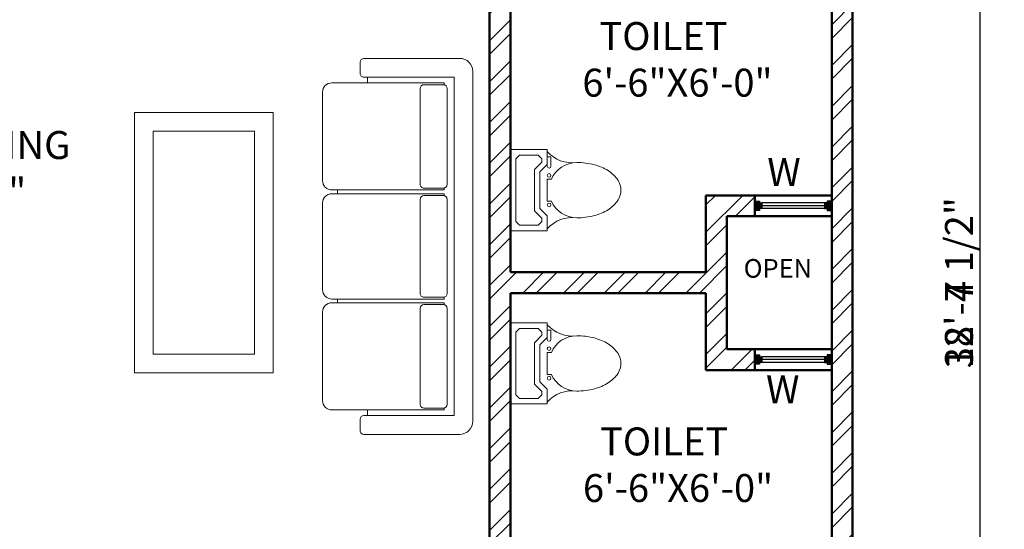
# Model space of a CAD drawing. Units: millimetres. Extents: x 4237 to 5109, y 21391 to 22486.
# Tile 15 of 17: x 4894 to 5105, y 22156 to 22265. Entities that reach past the tile are written whole.
import ezdxf

# ---------------------------------------------------------------- set-up
doc = ezdxf.new("R2010")
doc.units = ezdxf.units.MM
for name, color, linetype, lineweight in [('A-ANNO-DIMS', 2, 'Continuous', 18), ('A-ANNO-TEXT', 7, 'Continuous', 18), ('A-AREA-IDEN', 3, 'Continuous', 18), ('A-FURN', 8, 'Continuous', 18), ('A-WALL', 7, 'Continuous', 50), ('A-WALL-PATT', 252, 'Continuous', 13), ('windows', 140, 'Continuous', 25)]:
    doc.layers.add(name, color=color, linetype=linetype, lineweight=lineweight)
doc.styles.get("Standard").update_dxf_attribs({"font": 'arial.ttf'})
doc.dimstyles.new('ISO-25', dxfattribs={"dimtxt": 6, "dimasz": 2.5, "dimexe": 1.25, "dimexo": 0.625, "dimtad": 1, "dimdec": 1, "dimlunit": 4, "dimtxsty": 'Standard', "dimcen": 2.5, "dimadec": 0, "dimazin": 0, "dimtfac": 1, "dimtdec": 1, "dimtmove": 0, "dimatfit": 3, "dimfxl": 1, "dimarcsym": 0})

# ---------------------------------------------------------------- blocks, each defined once
blk = doc.blocks.new('A$C5EF6120A')
at = {"linetype": 'ByBlock'}
for p, q in [((0, 0.762), (0, 0.508)), ((0, 0.762), (0.5588, 0.762)), ((0.5588, 0.762), (0.5588, 0.508)), ((0.0381, 0.6985), (0.0635, 0.7239)), ((0.0381, 0.6985), (0.0381, 0.5715)), ((0.0635, 0.7239), (0.4953, 0.7239)), ((0.4953, 0.7239), (0.5207, 0.6985)), ((0.5207, 0.6985), (0.5207, 0.5715)), ((0.0635, 0.5461), (0.0381, 0.5715)), ((0.0635, 0.5461), (0.0858, 0.5461)), ((0.1366, 0.5969), (0.0858, 0.5461)), ((0.1524, 0.5588), (0.1016, 0.508)), ((0.1366, 0.5969), (0.4222, 0.5969)), ((0.1524, 0.5588), (0.4064, 0.5588)), ((0.4064, 0.5588), (0.4572, 0.508)), ((0.4222, 0.5969), (0.473, 0.5461)), ((0.4953, 0.5461), (0.473, 0.5461)), ((0.5207, 0.5715), (0.4953, 0.5461)), ((0, 0.508), (0.1016, 0.508)), ((0.0508, 0.508), (0.0508, 0.4826)), ((0.0508, 0.4826), (0.1143, 0.4826)), ((0.1143, 0.508), (0.1016, 0.508)), ((0.2032, 0.508), (0.2032, 0.4794)), ((0.3556, 0.508), (0.2032, 0.508)), ((0.3556, 0.508), (0.3556, 0.4794)), ((0.5588, 0.508), (0.4572, 0.508))]:
    blk.add_line(p, q, dxfattribs=at)
blk.add_lwpolyline([(0.0889, 0.3048, 0.063415), (0.1044, 0.183, 0.076468), (0.1447, 0.0893, 0.107136), (0.2118, 0.0204, 0.147373), (0.2794, 0, 0.147373), (0.347, 0.0204, 0.107136), (0.4141, 0.0893, 0.076468), (0.4544, 0.183, 0.063415), (0.4699, 0.3048, 0.063415)], format="xyb", dxfattribs=at)
for centre in [(0.1778, 0.4953), (0.381, 0.4953)]:
    blk.add_circle(centre, 0.0127, dxfattribs=at)
for centre, radius, start, end in [((-0.1375, 0.3358), 0.2285, 352.20108, 48.91101), ((0.2794, 0.3048), 0.1905, 113.57818, 180), ((0.1143, 0.4953), 0.0127, 270, 90), ((0.2794, 0.3048), 0.1905, 0, 66.42182), ((0.6963, 0.3358), 0.2285, 131.08899, 187.79892)]:
    blk.add_arc(centre, radius, start, end, dxfattribs=at)
blk = doc.blocks.new('A$C06FC73D7')
for p, q in [((1.93, 0.8), (0.07, 0.8)), ((0, 0.73), (0, 0.22)), ((0.1, 0.22), (0.1, 0.7)), ((0.1, 0.7), (1.9, 0.7)), ((1.9, 0.7), (1.9, 0.22)), ((2, 0.22), (2, 0.73)), ((0.13, 0.6479), (0.13, 0.05)), ((0.1404, 0.6479), (0.13, 0.6479)), ((0.14, 0.54), (0.14, 0.6437)), ((0.67, 0.6637), (0.16, 0.6637)), ((0.7, 0.6479), (0.6896, 0.6479)), ((0.69, 0.54), (0.69, 0.6437)), ((0.7, 0.05), (0.7, 0.6479)), ((0.72, 0.05), (0.72, 0.6479)), ((0.7304, 0.6479), (0.72, 0.6479)), ((0.73, 0.54), (0.73, 0.6437)), ((1.25, 0.6637), (0.75, 0.6637)), ((1.28, 0.6479), (1.2696, 0.6479)), ((1.27, 0.54), (1.27, 0.6437)), ((1.28, 0.05), (1.28, 0.6479)), ((1.3, 0.05), (1.3, 0.6479)), ((1.3104, 0.6479), (1.3, 0.6479)), ((1.31, 0.54), (1.31, 0.6437)), ((1.84, 0.6637), (1.33, 0.6637)), ((1.87, 0.6479), (1.86, 0.6479)), ((1.86, 0.54), (1.86, 0.6437)), ((1.87, 0.05), (1.87, 0.6479)), ((0.67, 0.52), (0.16, 0.52)), ((1.25, 0.52), (0.75, 0.52)), ((1.84, 0.52), (1.33, 0.52)), ((0.13, 0.24), (0.1, 0.24)), ((1.9, 0.24), (1.87, 0.24)), ((0.02, 0.2), (0.08, 0.2)), ((1.92, 0.2), (1.98, 0.2)), ((0.72, 0.08), (0.7, 0.08)), ((1.3, 0.08), (1.28, 0.08)), ((0.65, 0), (0.18, 0)), ((1.23, 0), (0.77, 0)), ((1.82, 0), (1.35, 0))]:
    blk.add_line(p, q)
for centre, radius, start, end in [((0.07, 0.73), 0.07, 90, 180), ((1.93, 0.73), 0.07, 0, 90), ((0.16, 0.6437), 0.02, 90, 180), ((0.67, 0.6437), 0.02, 0, 90), ((0.75, 0.6437), 0.02, 90, 180), ((1.25, 0.6437), 0.02, 0, 90), ((1.33, 0.6437), 0.02, 90, 180), ((1.84, 0.6437), 0.02, 0, 90), ((0.16, 0.54), 0.02, 180, 270), ((0.67, 0.54), 0.02, 270, 0), ((0.75, 0.54), 0.02, 180, 270), ((1.25, 0.54), 0.02, 270, 0), ((1.33, 0.54), 0.02, 180, 270), ((1.84, 0.54), 0.02, 270, 0), ((0.02, 0.22), 0.02, 180, 270), ((0.08, 0.22), 0.02, 270, 0), ((1.92, 0.22), 0.02, 180, 270), ((1.98, 0.22), 0.02, 270, 0), ((0.18, 0.05), 0.05, 180, 270), ((0.65, 0.05), 0.05, 270, 0), ((0.77, 0.05), 0.05, 180, 270), ((1.23, 0.05), 0.05, 270, 0), ((1.35, 0.05), 0.05, 180, 270), ((1.82, 0.05), 0.05, 270, 0)]:
    blk.add_arc(centre, radius, start, end)
blk = doc.blocks.new('*D116')
at = {"layer": 'A-ANNO-DIMS', "color": 0, "lineweight": -2, "transparency": 16777216}
for p, q in [((5073.14, 22440.7), (5101.11, 22440.7)), ((5099.86, 22438.2), (5099.86, 21979.7)), ((5073.14, 21977.2), (5101.11, 21977.2))]:
    blk.add_line(p, q, dxfattribs=at)
at = {"layer": 'A-ANNO-DIMS', "color": 0, "transparency": 16777216}
for points in [[(5099.45, 22438.2), (5100.28, 22438.2), (5099.86, 22440.7)], [(5099.45, 21979.7), (5100.28, 21979.7), (5099.86, 21977.2)]]:
    blk.add_solid(points, dxfattribs=at)
at = {"layer": 'Defpoints', "color": 0, "transparency": 16777216}
for p in [(5072.51, 22440.7), (5072.51, 21977.2), (5099.86, 21977.2)]:
    blk.add_point(p, dxfattribs=at)
at = {"layer": 'A-ANNO-DIMS', "color": 0, "transparency": 16777216, "insert": (5096.13, 22208.95), "char_height": 6, "attachment_point": 5, "rotation": 90}
blk.add_mtext('38\'-7 1/2"', dxfattribs=at)
blk = doc.blocks.new('*D118')
at = {"layer": 'A-ANNO-DIMS', "color": 0, "lineweight": -2, "transparency": 16777216}
for p, q in [((5068.64, 22283.2), (5101.11, 22283.2)), ((5099.86, 22280.7), (5099.86, 22137.2)), ((5064.14, 22134.7), (5101.11, 22134.7))]:
    blk.add_line(p, q, dxfattribs=at)
at = {"layer": 'A-ANNO-DIMS', "color": 0, "transparency": 16777216}
for points in [[(5099.45, 22280.7), (5100.28, 22280.7), (5099.86, 22283.2)], [(5099.45, 22137.2), (5100.28, 22137.2), (5099.86, 22134.7)]]:
    blk.add_solid(points, dxfattribs=at)
at = {"layer": 'Defpoints', "color": 0, "transparency": 16777216}
for p in [(5068.01, 22283.2), (5063.51, 22134.7), (5099.86, 22134.7)]:
    blk.add_point(p, dxfattribs=at)
at = {"layer": 'A-ANNO-DIMS', "color": 0, "transparency": 16777216, "insert": (5096.13, 22208.95), "char_height": 6, "attachment_point": 5, "rotation": 90}
blk.add_mtext('12\'-4 1/2"', dxfattribs=at)

msp = doc.modelspace()

# ---------------------------------------------------------------- hatches: boundary and pattern name
at = {"layer": 'A-WALL-PATT'}
h = msp.add_hatch(dxfattribs=at)
h.set_pattern_fill('ANSI32', color=256, scale=0.65)
h.paths.add_polyline_path([(5045.51, 22223.2), (5051.51, 22223.2), (5051.51, 22227.7), (5041.01, 22227.7), (5041.01, 22211.2), (4999.01, 22211.2), (4999.01, 22283.2), (5017.01, 22283.2), (5017.01, 22287.7), (4965.41, 22287.7), (4965.41, 22283.2), (4994.51, 22283.2), (4994.51, 22134.7), (4938.41, 22134.7), (4938.41, 22130.2), (5011.33, 22130.2), (5011.33, 22134.7), (4999.01, 22134.7), (4999.01, 22206.7), (5041.01, 22206.7), (5041.01, 22190.2), (5051.51, 22190.2), (5051.51, 22194.7), (5045.51, 22194.7)])
h = msp.add_hatch(dxfattribs=at)
h.set_pattern_fill('ANSI32', color=256, scale=0.65)
h.paths.add_polyline_path([(5072.51, 22283.2), (5068.01, 22283.2), (5068.01, 22144), (5072.51, 22144)])
h = msp.add_hatch(color=256, dxfattribs=at)
h.dxf.hatch_style = 1
h.paths.add_polyline_path([(5052.51, 22224.45), (5052.51, 22224.84), (5053.03, 22224.84), (5053.03, 22226.06), (5052.51, 22226.06), (5052.51, 22226.45), (5051.51, 22226.45), (5051.51, 22224.45)])
h = msp.add_hatch(color=256, dxfattribs=at)
h.dxf.hatch_style = 1
h.paths.add_polyline_path([(5067.01, 22224.84), (5067.01, 22224.45), (5068.01, 22224.45), (5068.01, 22226.45), (5067.01, 22226.45), (5067.01, 22226.06), (5066.5, 22226.06), (5066.5, 22224.84)])
h = msp.add_hatch(color=256, dxfattribs=at)
h.dxf.hatch_style = 1
h.paths.add_polyline_path([(5052.51, 22191.45), (5052.51, 22191.84), (5053.03, 22191.84), (5053.03, 22193.06), (5052.51, 22193.06), (5052.51, 22193.45), (5051.51, 22193.45), (5051.51, 22191.45)])
h = msp.add_hatch(color=256, dxfattribs=at)
h.dxf.hatch_style = 1
h.paths.add_polyline_path([(5067.01, 22191.84), (5067.01, 22191.45), (5068.01, 22191.45), (5068.01, 22193.45), (5067.01, 22193.45), (5067.01, 22193.06), (5066.5, 22193.06), (5066.5, 22191.84)])

# ---------------------------------------------------------------- linework, layer by layer
at = {"layer": 'A-FURN'}
for points in [[(4918.26, 22245.5), (4948.06, 22245.5), (4948.06, 22189.61), (4918.26, 22189.61)], [(4922.26, 22241.5), (4944.06, 22241.5), (4944.06, 22193.61), (4922.26, 22193.61)]]:
    msp.add_lwpolyline(points, close=True, dxfattribs=at)
at = {"layer": 'A-WALL'}
for p, q in [((5072.51, 22436.2), (5072.51, 21977.2)), ((4994.51, 22283.2), (4994.51, 22134.7)), ((4999.01, 22283.2), (4999.01, 22211.2)), ((5068.01, 22283.2), (5068.01, 22144)), ((5041.01, 22227.7), (5041.01, 22211.2)), ((5041.01, 22227.7), (5068.01, 22227.7)), ((5051.51, 22227.7), (5051.51, 22223.2)), ((5045.51, 22223.2), (5045.51, 22194.7)), ((5045.51, 22223.2), (5068.01, 22223.2)), ((4999.01, 22211.2), (5041.01, 22211.2)), ((4999.01, 22206.7), (5041.01, 22206.7)), ((4999.01, 22206.7), (4999.01, 22134.7)), ((5041.01, 22206.7), (5041.01, 22190.2)), ((5045.51, 22194.7), (5068.01, 22194.7)), ((5051.51, 22194.7), (5051.51, 22190.2)), ((5041.01, 22190.2), (5068.01, 22190.2))]:
    msp.add_line(p, q, dxfattribs=at)
at = {"layer": 'windows'}
for p, q in [((5066.5, 22226.06), (5053.03, 22226.06)), ((5066.5, 22225.45), (5053.03, 22225.45)), ((5066.5, 22224.84), (5053.03, 22224.84)), ((5066.5, 22193.06), (5053.03, 22193.06)), ((5066.5, 22192.45), (5053.03, 22192.45)), ((5066.5, 22191.84), (5053.03, 22191.84))]:
    msp.add_line(p, q, dxfattribs=at)
for points in [[(5068.01, 22227.7), (5068.01, 22223.2), (5051.51, 22223.2), (5051.51, 22227.7)], [(5068.01, 22194.7), (5068.01, 22190.2), (5051.51, 22190.2), (5051.51, 22194.7)]]:
    msp.add_lwpolyline(points, close=True, dxfattribs=at)
for points in [[(5051.51, 22226.45), (5052.51, 22226.45), (5052.51, 22226.06), (5053.03, 22226.06), (5053.03, 22224.84), (5052.51, 22224.84), (5052.51, 22224.45), (5051.51, 22224.45)], [(5068.01, 22226.45), (5067.01, 22226.45), (5067.01, 22226.06), (5066.5, 22226.06), (5066.5, 22224.84), (5067.01, 22224.84), (5067.01, 22224.45), (5068.01, 22224.45)], [(5051.51, 22193.45), (5052.51, 22193.45), (5052.51, 22193.06), (5053.03, 22193.06), (5053.03, 22191.84), (5052.51, 22191.84), (5052.51, 22191.45), (5051.51, 22191.45)], [(5068.01, 22193.45), (5067.01, 22193.45), (5067.01, 22193.06), (5066.5, 22193.06), (5066.5, 22191.84), (5067.01, 22191.84), (5067.01, 22191.45), (5068.01, 22191.45)]]:
    msp.add_lwpolyline(points, dxfattribs=at)

# ---------------------------------------------------------------- block references
at = {"layer": 'A-FURN'}
for name, p, xscale, yscale, zscale, rotation in [('A$C06FC73D7', (4958.66, 22257.1), 40.35424995786203, 40.35424995786203, 40.35424995786203, 270), ('A$C5EF6120A', (5022.76, 22237.52), -31.17096342775826, 31.17096342775826, 31.17096342775826, 90), ('A$C5EF6120A', (5022.76, 22200.33), -31.17096342775826, 31.17096342775826, 31.17096342775826, 90)]:
    msp.add_blockref(name, p, dxfattribs=dict(at, xscale=xscale, yscale=yscale, zscale=zscale, rotation=rotation))

# ---------------------------------------------------------------- texts
at = {"layer": 'A-ANNO-TEXT', "attachment_point": 1}
for s, width, insert, char_height in [('    W', 21.7253, (5046.84, 22235.72), 6), ('  OPEN', 28.9883, (5046.67, 22214.02), 4), ('    W', 21.7253, (5046.57, 22189.07), 6)]:
    msp.add_mtext_dynamic_manual_height_columns(s, width=width, gutter_width=12.5, heights=[0], dxfattribs=dict(at, insert=insert, char_height=char_height))
at = {"layer": 'A-AREA-IDEN', "char_height": 6, "attachment_point": 1}
for s, width, insert in [('     TOILET\\P   6\'-6"X6\'-0"', 55.7646, (5008.96, 22264.89)), (' DRAWING / DINING  \\P    16\'-1.8"X12\'-3"                ', 94.8365, (4830.95, 22241.5)), ('     TOILET\\P   6\'-6"X6\'-0"', 55.7646, (5009.09, 22177.87))]:
    msp.add_mtext_dynamic_manual_height_columns(s, width=width, gutter_width=12.5, heights=[0], dxfattribs=dict(at, insert=insert))

# ---------------------------------------------------------------- dimensions: what is measured, and where the dimension line sits
at = {"layer": 'A-ANNO-DIMS'}
for base, p1, p2, picture in [((5099.86, 21977.2), (5072.51, 22440.7), (5072.51, 21977.2), '*D116'), ((5099.86, 22134.7), (5068.01, 22283.2), (5063.51, 22134.7), '*D118')]:
    dim = msp.add_linear_dim(base=base, p1=p1, p2=p2, angle=90, dimstyle='ISO-25', override={"dimdec": 1, "dimlfac": 1, "dimrnd": 0, "dimzin": 1, "dimdsep": 46, "dimlunit": 4, "dimfrac": 2}, dxfattribs=at)
    dim.commit()
    dim.dimension.update_dxf_attribs({"geometry": picture, "text_midpoint": (5096.13, 22208.95)})

doc.saveas('drawing.dxf')
